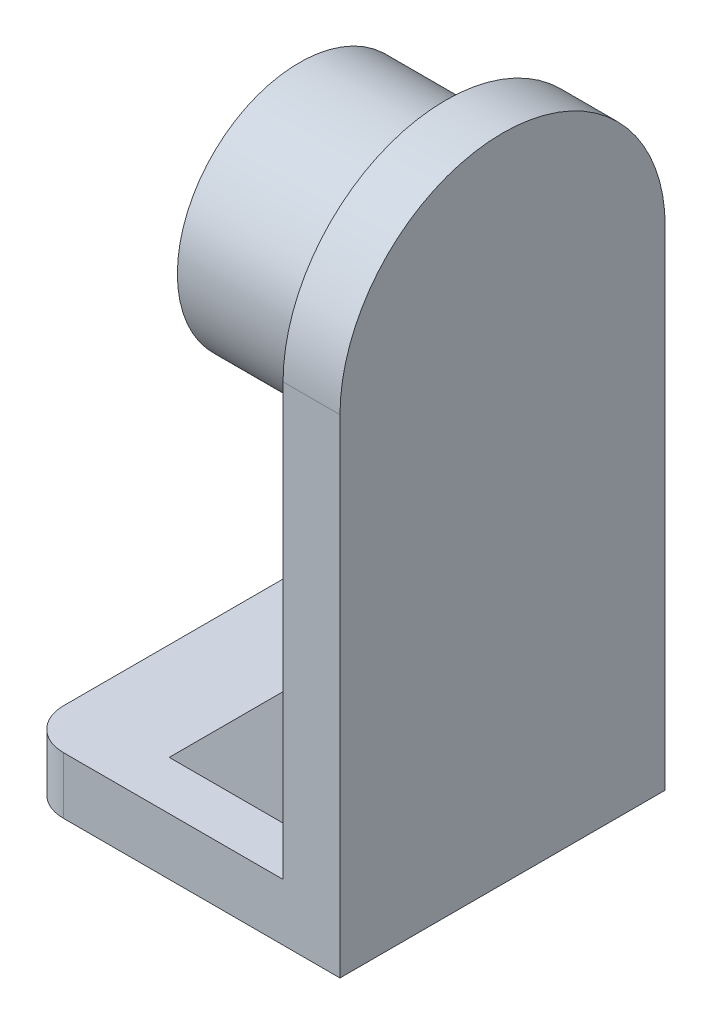
ISO-10303-21;
HEADER;
FILE_DESCRIPTION(('STEP AP214'),'2;1');
FILE_NAME('part.step','',(''),(''),'','','');
FILE_SCHEMA(('AUTOMOTIVE_DESIGN { 1 0 10303 214 1 1 1 1 }'));
ENDSEC;
DATA;
#1=APPLICATION_CONTEXT('core data for automotive mechanical design processes');
#2=APPLICATION_PROTOCOL_DEFINITION('international standard','automotive_design',2000,#1);
#3=PRODUCT_CONTEXT('',#1,'mechanical');
#4=PRODUCT('Part','Part','',(#3));
#5=PRODUCT_RELATED_PRODUCT_CATEGORY('part','',(#4));
#6=PRODUCT_DEFINITION_FORMATION('','',#4);
#7=PRODUCT_DEFINITION_CONTEXT('part definition',#1,'design');
#8=PRODUCT_DEFINITION('design','',#6,#7);
#9=PRODUCT_DEFINITION_SHAPE('','',#8);
#10=(LENGTH_UNIT() NAMED_UNIT(*) SI_UNIT(.MILLI.,.METRE.));
#11=(NAMED_UNIT(*) PLANE_ANGLE_UNIT() SI_UNIT($,.RADIAN.));
#12=(NAMED_UNIT(*) SI_UNIT($,.STERADIAN.) SOLID_ANGLE_UNIT());
#13=UNCERTAINTY_MEASURE_WITH_UNIT(LENGTH_MEASURE(1.E-05),#10,'distance_accuracy_value','');
#14=(GEOMETRIC_REPRESENTATION_CONTEXT(3) GLOBAL_UNCERTAINTY_ASSIGNED_CONTEXT((#13)) GLOBAL_UNIT_ASSIGNED_CONTEXT((#10,
#11,#12)) REPRESENTATION_CONTEXT('',''));
#15=CARTESIAN_POINT('',(0.,0.,0.));
#16=DIRECTION('',(0.,0.,1.));
#17=DIRECTION('',(1.,0.,0.));
#18=AXIS2_PLACEMENT_3D('',#15,#16,#17);
#19=CARTESIAN_POINT('',(7.,7.,12.));
#20=DIRECTION('',(-0.707106781186547,0.707106781186548,0.));
#21=DIRECTION('',(-0.707106781186548,-0.707106781186547,0.));
#22=AXIS2_PLACEMENT_3D('',#19,#20,#21);
#23=PLANE('',#22);
#24=DIRECTION('',(0.,0.,-1.));
#25=VECTOR('',#24,1.);
#26=CARTESIAN_POINT('',(27.,27.,12.));
#27=LINE('',#26,#25);
#28=CARTESIAN_POINT('',(27.,27.,12.));
#29=VERTEX_POINT('',#28);
#30=CARTESIAN_POINT('',(27.,27.,6.));
#31=VERTEX_POINT('',#30);
#32=EDGE_CURVE('E276',#29,#31,#27,.T.);
#33=ORIENTED_EDGE('',*,*,#32,.T.);
#34=DIRECTION('',(0.707106781186548,0.707106781186548,0.));
#35=VECTOR('',#34,1.);
#36=CARTESIAN_POINT('',(27.,27.,6.));
#37=LINE('',#36,#35);
#38=CARTESIAN_POINT('',(7.,7.,6.));
#39=VERTEX_POINT('',#38);
#40=EDGE_CURVE('E267',#39,#31,#37,.T.);
#41=ORIENTED_EDGE('',*,*,#40,.F.);
#42=DIRECTION('',(0.,0.,-1.));
#43=VECTOR('',#42,1.);
#44=CARTESIAN_POINT('',(7.,7.,12.));
#45=LINE('',#44,#43);
#46=CARTESIAN_POINT('',(7.,7.,12.));
#47=VERTEX_POINT('',#46);
#48=EDGE_CURVE('E279',#47,#39,#45,.T.);
#49=ORIENTED_EDGE('',*,*,#48,.F.);
#50=DIRECTION('',(0.707106781186548,0.707106781186547,0.));
#51=VECTOR('',#50,1.);
#52=CARTESIAN_POINT('',(7.,7.,12.));
#53=LINE('',#52,#51);
#54=EDGE_CURVE('E273',#47,#29,#53,.T.);
#55=ORIENTED_EDGE('',*,*,#54,.T.);
#56=EDGE_LOOP('',(#33,#41,#49,#55));
#57=FACE_BOUND('',#56,.T.);
#58=ADVANCED_FACE('F44',(#57),#23,.T.);
#59=CARTESIAN_POINT('',(0.,0.,40.));
#60=DIRECTION('',(0.,1.,0.));
#61=DIRECTION('',(0.,0.,1.));
#62=AXIS2_PLACEMENT_3D('',#59,#60,#61);
#63=PLANE('',#62);
#64=DIRECTION('',(1.,0.,0.));
#65=VECTOR('',#64,1.);
#66=CARTESIAN_POINT('',(0.,0.,0.));
#67=LINE('',#66,#65);
#68=CARTESIAN_POINT('',(0.,0.,0.));
#69=VERTEX_POINT('',#68);
#70=CARTESIAN_POINT('',(34.,0.,0.));
#71=VERTEX_POINT('',#70);
#72=EDGE_CURVE('E226',#69,#71,#67,.T.);
#73=ORIENTED_EDGE('',*,*,#72,.T.);
#74=DIRECTION('',(0.,0.,-1.));
#75=VECTOR('',#74,1.);
#76=CARTESIAN_POINT('',(34.,0.,40.));
#77=LINE('',#76,#75);
#78=CARTESIAN_POINT('',(34.,0.,40.));
#79=VERTEX_POINT('',#78);
#80=EDGE_CURVE('E52',#79,#71,#77,.T.);
#81=ORIENTED_EDGE('',*,*,#80,.F.);
#82=DIRECTION('',(1.,0.,0.));
#83=VECTOR('',#82,1.);
#84=CARTESIAN_POINT('',(0.,0.,40.));
#85=LINE('',#84,#83);
#86=CARTESIAN_POINT('',(0.,0.,40.));
#87=VERTEX_POINT('',#86);
#88=EDGE_CURVE('E211',#87,#79,#85,.T.);
#89=ORIENTED_EDGE('',*,*,#88,.F.);
#90=CARTESIAN_POINT('',(0.,0.,35.));
#91=DIRECTION('',(0.,1.,0.));
#92=DIRECTION('',(0.,0.,1.));
#93=AXIS2_PLACEMENT_3D('',#90,#91,#92);
#94=CIRCLE('',#93,5.);
#95=CARTESIAN_POINT('',(-5.,0.,35.));
#96=VERTEX_POINT('',#95);
#97=EDGE_CURVE('E196',#96,#87,#94,.T.);
#98=ORIENTED_EDGE('',*,*,#97,.F.);
#99=DIRECTION('',(0.,0.,1.));
#100=VECTOR('',#99,1.);
#101=CARTESIAN_POINT('',(-5.,0.,5.));
#102=LINE('',#101,#100);
#103=CARTESIAN_POINT('',(-5.,0.,5.));
#104=VERTEX_POINT('',#103);
#105=EDGE_CURVE('E195',#104,#96,#102,.T.);
#106=ORIENTED_EDGE('',*,*,#105,.F.);
#107=CARTESIAN_POINT('',(0.,0.,5.));
#108=DIRECTION('',(0.,1.,0.));
#109=DIRECTION('',(0.,0.,1.));
#110=AXIS2_PLACEMENT_3D('',#107,#108,#109);
#111=CIRCLE('',#110,5.);
#112=EDGE_CURVE('E186',#69,#104,#111,.T.);
#113=ORIENTED_EDGE('',*,*,#112,.F.);
#114=EDGE_LOOP('',(#73,#81,#89,#98,#106,#113));
#115=FACE_BOUND('',#114,.T.);
#116=ADVANCED_FACE('F50',(#115),#63,.F.);
#117=CARTESIAN_POINT('',(34.,0.,40.));
#118=DIRECTION('',(-1.,0.,0.));
#119=DIRECTION('',(0.,0.,1.));
#120=AXIS2_PLACEMENT_3D('',#117,#118,#119);
#121=PLANE('',#120);
#122=DIRECTION('',(0.,1.,0.));
#123=VECTOR('',#122,1.);
#124=CARTESIAN_POINT('',(34.,0.,0.));
#125=LINE('',#124,#123);
#126=CARTESIAN_POINT('',(34.,60.,0.));
#127=VERTEX_POINT('',#126);
#128=EDGE_CURVE('E229',#71,#127,#125,.T.);
#129=ORIENTED_EDGE('',*,*,#128,.T.);
#130=CARTESIAN_POINT('',(34.,60.,20.));
#131=DIRECTION('',(-1.,0.,0.));
#132=DIRECTION('',(0.,0.,1.));
#133=AXIS2_PLACEMENT_3D('',#130,#131,#132);
#134=CIRCLE('',#133,20.);
#135=CARTESIAN_POINT('',(34.,60.,40.));
#136=VERTEX_POINT('',#135);
#137=EDGE_CURVE('E182',#136,#127,#134,.T.);
#138=ORIENTED_EDGE('',*,*,#137,.F.);
#139=DIRECTION('',(0.,1.,0.));
#140=VECTOR('',#139,1.);
#141=CARTESIAN_POINT('',(34.,0.,40.));
#142=LINE('',#141,#140);
#143=EDGE_CURVE('E217',#79,#136,#142,.T.);
#144=ORIENTED_EDGE('',*,*,#143,.F.);
#145=ORIENTED_EDGE('',*,*,#80,.T.);
#146=EDGE_LOOP('',(#129,#138,#144,#145));
#147=FACE_BOUND('',#146,.T.);
#148=ADVANCED_FACE('F242',(#147),#121,.F.);
#149=CARTESIAN_POINT('',(27.,7.,40.));
#150=DIRECTION('',(1.,0.,0.));
#151=DIRECTION('',(0.,0.,-1.));
#152=AXIS2_PLACEMENT_3D('',#149,#150,#151);
#153=PLANE('',#152);
#154=CARTESIAN_POINT('',(27.,60.,20.));
#155=DIRECTION('',(1.,0.,0.));
#156=DIRECTION('',(0.,0.,-1.));
#157=AXIS2_PLACEMENT_3D('',#154,#155,#156);
#158=CIRCLE('',#157,15.);
#159=CARTESIAN_POINT('',(27.,60.,5.));
#160=VERTEX_POINT('',#159);
#161=EDGE_CURVE('E11',#160,#160,#158,.F.);
#162=ORIENTED_EDGE('',*,*,#161,.F.);
#163=EDGE_LOOP('',(#162));
#164=FACE_BOUND('',#163,.T.);
#165=DIRECTION('',(0.,-1.,0.));
#166=VECTOR('',#165,1.);
#167=CARTESIAN_POINT('',(27.,7.,0.));
#168=LINE('',#167,#166);
#169=CARTESIAN_POINT('',(27.,60.,0.));
#170=VERTEX_POINT('',#169);
#171=CARTESIAN_POINT('',(27.,7.,0.));
#172=VERTEX_POINT('',#171);
#173=EDGE_CURVE('E232',#170,#172,#168,.T.);
#174=ORIENTED_EDGE('',*,*,#173,.T.);
#175=DIRECTION('',(0.,0.,-1.));
#176=VECTOR('',#175,1.);
#177=CARTESIAN_POINT('',(27.,7.,6.));
#178=LINE('',#177,#176);
#179=CARTESIAN_POINT('',(27.,7.,6.));
#180=VERTEX_POINT('',#179);
#181=EDGE_CURVE('E269',#180,#172,#178,.T.);
#182=ORIENTED_EDGE('',*,*,#181,.F.);
#183=DIRECTION('',(0.,-1.,0.));
#184=VECTOR('',#183,1.);
#185=CARTESIAN_POINT('',(27.,7.,6.));
#186=LINE('',#185,#184);
#187=EDGE_CURVE('E261',#31,#180,#186,.T.);
#188=ORIENTED_EDGE('',*,*,#187,.F.);
#189=ORIENTED_EDGE('',*,*,#32,.F.);
#190=DIRECTION('',(0.,-1.,0.));
#191=VECTOR('',#190,1.);
#192=CARTESIAN_POINT('',(27.,27.,12.));
#193=LINE('',#192,#191);
#194=CARTESIAN_POINT('',(27.,7.,12.));
#195=VERTEX_POINT('',#194);
#196=EDGE_CURVE('E272',#29,#195,#193,.T.);
#197=ORIENTED_EDGE('',*,*,#196,.T.);
#198=DIRECTION('',(0.,0.,-1.));
#199=VECTOR('',#198,1.);
#200=CARTESIAN_POINT('',(27.,7.,40.));
#201=LINE('',#200,#199);
#202=CARTESIAN_POINT('',(27.,7.,28.));
#203=VERTEX_POINT('',#202);
#204=EDGE_CURVE('E223',#203,#195,#201,.T.);
#205=ORIENTED_EDGE('',*,*,#204,.F.);
#206=DIRECTION('',(0.,1.,0.));
#207=VECTOR('',#206,1.);
#208=CARTESIAN_POINT('',(27.,7.,28.));
#209=LINE('',#208,#207);
#210=CARTESIAN_POINT('',(27.,27.,28.));
#211=VERTEX_POINT('',#210);
#212=EDGE_CURVE('E285',#203,#211,#209,.T.);
#213=ORIENTED_EDGE('',*,*,#212,.T.);
#214=DIRECTION('',(0.,0.,1.));
#215=VECTOR('',#214,1.);
#216=CARTESIAN_POINT('',(27.,27.,28.));
#217=LINE('',#216,#215);
#218=CARTESIAN_POINT('',(27.,27.,34.));
#219=VERTEX_POINT('',#218);
#220=EDGE_CURVE('E166',#211,#219,#217,.T.);
#221=ORIENTED_EDGE('',*,*,#220,.T.);
#222=DIRECTION('',(0.,1.,0.));
#223=VECTOR('',#222,1.);
#224=CARTESIAN_POINT('',(27.,7.,34.));
#225=LINE('',#224,#223);
#226=CARTESIAN_POINT('',(27.,7.,34.));
#227=VERTEX_POINT('',#226);
#228=EDGE_CURVE('E58',#227,#219,#225,.T.);
#229=ORIENTED_EDGE('',*,*,#228,.F.);
#230=DIRECTION('',(0.,0.,1.));
#231=VECTOR('',#230,1.);
#232=CARTESIAN_POINT('',(27.,7.,34.));
#233=LINE('',#232,#231);
#234=CARTESIAN_POINT('',(27.,7.,40.));
#235=VERTEX_POINT('',#234);
#236=EDGE_CURVE('E163',#227,#235,#233,.T.);
#237=ORIENTED_EDGE('',*,*,#236,.T.);
#238=DIRECTION('',(0.,-1.,0.));
#239=VECTOR('',#238,1.);
#240=CARTESIAN_POINT('',(27.,7.,40.));
#241=LINE('',#240,#239);
#242=CARTESIAN_POINT('',(27.,60.,40.));
#243=VERTEX_POINT('',#242);
#244=EDGE_CURVE('E222',#243,#235,#241,.T.);
#245=ORIENTED_EDGE('',*,*,#244,.F.);
#246=CARTESIAN_POINT('',(27.,60.,20.));
#247=DIRECTION('',(-1.,0.,0.));
#248=DIRECTION('',(0.,0.,1.));
#249=AXIS2_PLACEMENT_3D('',#246,#247,#248);
#250=CIRCLE('',#249,20.);
#251=EDGE_CURVE('E185',#243,#170,#250,.T.);
#252=ORIENTED_EDGE('',*,*,#251,.T.);
#253=EDGE_LOOP('',(#174,#182,#188,#189,#197,#205,#213,#221,#229,#237,#245,#252));
#254=FACE_BOUND('',#253,.T.);
#255=ADVANCED_FACE('F258',(#164,#254),#153,.F.);
#256=CARTESIAN_POINT('',(0.,7.,40.));
#257=DIRECTION('',(0.,-1.,0.));
#258=DIRECTION('',(0.,0.,-1.));
#259=AXIS2_PLACEMENT_3D('',#256,#257,#258);
#260=PLANE('',#259);
#261=DIRECTION('',(-1.,0.,0.));
#262=VECTOR('',#261,1.);
#263=CARTESIAN_POINT('',(27.,7.,12.));
#264=LINE('',#263,#262);
#265=EDGE_CURVE('E271',#195,#47,#264,.T.);
#266=ORIENTED_EDGE('',*,*,#265,.T.);
#267=ORIENTED_EDGE('',*,*,#48,.T.);
#268=DIRECTION('',(-1.,0.,0.));
#269=VECTOR('',#268,1.);
#270=CARTESIAN_POINT('',(7.,7.,6.));
#271=LINE('',#270,#269);
#272=EDGE_CURVE('E69',#180,#39,#271,.T.);
#273=ORIENTED_EDGE('',*,*,#272,.F.);
#274=ORIENTED_EDGE('',*,*,#181,.T.);
#275=DIRECTION('',(-1.,0.,0.));
#276=VECTOR('',#275,1.);
#277=CARTESIAN_POINT('',(0.,7.,0.));
#278=LINE('',#277,#276);
#279=CARTESIAN_POINT('',(0.,7.,0.));
#280=VERTEX_POINT('',#279);
#281=EDGE_CURVE('E213',#172,#280,#278,.T.);
#282=ORIENTED_EDGE('',*,*,#281,.T.);
#283=CARTESIAN_POINT('',(0.,7.,5.));
#284=DIRECTION('',(0.,1.,0.));
#285=DIRECTION('',(0.,0.,1.));
#286=AXIS2_PLACEMENT_3D('',#283,#284,#285);
#287=CIRCLE('',#286,5.);
#288=CARTESIAN_POINT('',(-5.,7.,5.));
#289=VERTEX_POINT('',#288);
#290=EDGE_CURVE('E187',#280,#289,#287,.T.);
#291=ORIENTED_EDGE('',*,*,#290,.T.);
#292=DIRECTION('',(0.,0.,1.));
#293=VECTOR('',#292,1.);
#294=CARTESIAN_POINT('',(-5.,7.,5.));
#295=LINE('',#294,#293);
#296=CARTESIAN_POINT('',(-5.,7.,35.));
#297=VERTEX_POINT('',#296);
#298=EDGE_CURVE('E205',#289,#297,#295,.T.);
#299=ORIENTED_EDGE('',*,*,#298,.T.);
#300=CARTESIAN_POINT('',(0.,7.,35.));
#301=DIRECTION('',(0.,1.,0.));
#302=DIRECTION('',(0.,0.,1.));
#303=AXIS2_PLACEMENT_3D('',#300,#301,#302);
#304=CIRCLE('',#303,5.);
#305=CARTESIAN_POINT('',(0.,7.,40.));
#306=VERTEX_POINT('',#305);
#307=EDGE_CURVE('E194',#297,#306,#304,.T.);
#308=ORIENTED_EDGE('',*,*,#307,.T.);
#309=DIRECTION('',(-1.,0.,0.));
#310=VECTOR('',#309,1.);
#311=CARTESIAN_POINT('',(0.,7.,40.));
#312=LINE('',#311,#310);
#313=EDGE_CURVE('E224',#235,#306,#312,.T.);
#314=ORIENTED_EDGE('',*,*,#313,.F.);
#315=ORIENTED_EDGE('',*,*,#236,.F.);
#316=DIRECTION('',(1.,0.,0.));
#317=VECTOR('',#316,1.);
#318=CARTESIAN_POINT('',(7.,7.,34.));
#319=LINE('',#318,#317);
#320=CARTESIAN_POINT('',(7.,7.,34.));
#321=VERTEX_POINT('',#320);
#322=EDGE_CURVE('E146',#321,#227,#319,.T.);
#323=ORIENTED_EDGE('',*,*,#322,.F.);
#324=DIRECTION('',(0.,0.,1.));
#325=VECTOR('',#324,1.);
#326=CARTESIAN_POINT('',(7.,7.,28.));
#327=LINE('',#326,#325);
#328=CARTESIAN_POINT('',(7.,7.,28.));
#329=VERTEX_POINT('',#328);
#330=EDGE_CURVE('E159',#329,#321,#327,.T.);
#331=ORIENTED_EDGE('',*,*,#330,.F.);
#332=DIRECTION('',(1.,0.,0.));
#333=VECTOR('',#332,1.);
#334=CARTESIAN_POINT('',(27.,7.,28.));
#335=LINE('',#334,#333);
#336=EDGE_CURVE('E282',#329,#203,#335,.T.);
#337=ORIENTED_EDGE('',*,*,#336,.T.);
#338=ORIENTED_EDGE('',*,*,#204,.T.);
#339=EDGE_LOOP('',(#266,#267,#273,#274,#282,#291,#299,#308,#314,#315,#323,#331,#337,#338));
#340=FACE_BOUND('',#339,.T.);
#341=ADVANCED_FACE('F157',(#340),#260,.F.);
#342=CARTESIAN_POINT('',(0.,0.,40.));
#343=DIRECTION('',(0.,0.,-1.));
#344=DIRECTION('',(-1.,0.,0.));
#345=AXIS2_PLACEMENT_3D('',#342,#343,#344);
#346=PLANE('',#345);
#347=ORIENTED_EDGE('',*,*,#244,.T.);
#348=ORIENTED_EDGE('',*,*,#313,.T.);
#349=DIRECTION('',(0.,-1.,0.));
#350=VECTOR('',#349,1.);
#351=CARTESIAN_POINT('',(0.,0.,40.));
#352=LINE('',#351,#350);
#353=EDGE_CURVE('E212',#306,#87,#352,.T.);
#354=ORIENTED_EDGE('',*,*,#353,.T.);
#355=ORIENTED_EDGE('',*,*,#88,.T.);
#356=ORIENTED_EDGE('',*,*,#143,.T.);
#357=DIRECTION('',(-1.,0.,0.));
#358=VECTOR('',#357,1.);
#359=CARTESIAN_POINT('',(34.,60.,40.));
#360=LINE('',#359,#358);
#361=EDGE_CURVE('E218',#136,#243,#360,.T.);
#362=ORIENTED_EDGE('',*,*,#361,.T.);
#363=EDGE_LOOP('',(#347,#348,#354,#355,#356,#362));
#364=FACE_BOUND('',#363,.T.);
#365=ADVANCED_FACE('F259',(#364),#346,.F.);
#366=CARTESIAN_POINT('',(0.,0.,0.));
#367=DIRECTION('',(0.,0.,-1.));
#368=DIRECTION('',(-1.,0.,0.));
#369=AXIS2_PLACEMENT_3D('',#366,#367,#368);
#370=PLANE('',#369);
#371=ORIENTED_EDGE('',*,*,#281,.F.);
#372=ORIENTED_EDGE('',*,*,#173,.F.);
#373=DIRECTION('',(-1.,0.,0.));
#374=VECTOR('',#373,1.);
#375=CARTESIAN_POINT('',(34.,60.,0.));
#376=LINE('',#375,#374);
#377=EDGE_CURVE('E235',#127,#170,#376,.T.);
#378=ORIENTED_EDGE('',*,*,#377,.F.);
#379=ORIENTED_EDGE('',*,*,#128,.F.);
#380=ORIENTED_EDGE('',*,*,#72,.F.);
#381=DIRECTION('',(0.,-1.,0.));
#382=VECTOR('',#381,1.);
#383=CARTESIAN_POINT('',(0.,0.,0.));
#384=LINE('',#383,#382);
#385=EDGE_CURVE('E209',#280,#69,#384,.T.);
#386=ORIENTED_EDGE('',*,*,#385,.F.);
#387=EDGE_LOOP('',(#371,#372,#378,#379,#380,#386));
#388=FACE_BOUND('',#387,.T.);
#389=ADVANCED_FACE('F249',(#388),#370,.T.);
#390=CARTESIAN_POINT('',(0.,0.,5.));
#391=DIRECTION('',(0.,1.,0.));
#392=DIRECTION('',(0.,0.,1.));
#393=AXIS2_PLACEMENT_3D('',#390,#391,#392);
#394=CYLINDRICAL_SURFACE('',#393,5.);
#395=ORIENTED_EDGE('',*,*,#290,.F.);
#396=ORIENTED_EDGE('',*,*,#385,.T.);
#397=ORIENTED_EDGE('',*,*,#112,.T.);
#398=DIRECTION('',(0.,1.,0.));
#399=VECTOR('',#398,1.);
#400=CARTESIAN_POINT('',(-5.,0.,5.));
#401=LINE('',#400,#399);
#402=EDGE_CURVE('E198',#104,#289,#401,.T.);
#403=ORIENTED_EDGE('',*,*,#402,.T.);
#404=EDGE_LOOP('',(#395,#396,#397,#403));
#405=FACE_BOUND('',#404,.T.);
#406=ADVANCED_FACE('F301',(#405),#394,.T.);
#407=CARTESIAN_POINT('',(0.,0.,35.));
#408=DIRECTION('',(0.,1.,0.));
#409=DIRECTION('',(0.,0.,1.));
#410=AXIS2_PLACEMENT_3D('',#407,#408,#409);
#411=CYLINDRICAL_SURFACE('',#410,5.);
#412=ORIENTED_EDGE('',*,*,#307,.F.);
#413=DIRECTION('',(0.,1.,0.));
#414=VECTOR('',#413,1.);
#415=CARTESIAN_POINT('',(-5.,0.,35.));
#416=LINE('',#415,#414);
#417=EDGE_CURVE('E210',#96,#297,#416,.T.);
#418=ORIENTED_EDGE('',*,*,#417,.F.);
#419=ORIENTED_EDGE('',*,*,#97,.T.);
#420=ORIENTED_EDGE('',*,*,#353,.F.);
#421=EDGE_LOOP('',(#412,#418,#419,#420));
#422=FACE_BOUND('',#421,.T.);
#423=ADVANCED_FACE('F309',(#422),#411,.T.);
#424=CARTESIAN_POINT('',(-5.,0.,5.));
#425=DIRECTION('',(-1.,0.,0.));
#426=DIRECTION('',(0.,0.,1.));
#427=AXIS2_PLACEMENT_3D('',#424,#425,#426);
#428=PLANE('',#427);
#429=ORIENTED_EDGE('',*,*,#298,.F.);
#430=ORIENTED_EDGE('',*,*,#402,.F.);
#431=ORIENTED_EDGE('',*,*,#105,.T.);
#432=ORIENTED_EDGE('',*,*,#417,.T.);
#433=EDGE_LOOP('',(#429,#430,#431,#432));
#434=FACE_BOUND('',#433,.T.);
#435=ADVANCED_FACE('F304',(#434),#428,.T.);
#436=CARTESIAN_POINT('',(34.,60.,20.));
#437=DIRECTION('',(-1.,0.,0.));
#438=DIRECTION('',(0.,0.,1.));
#439=AXIS2_PLACEMENT_3D('',#436,#437,#438);
#440=CYLINDRICAL_SURFACE('',#439,20.);
#441=ORIENTED_EDGE('',*,*,#251,.F.);
#442=ORIENTED_EDGE('',*,*,#361,.F.);
#443=ORIENTED_EDGE('',*,*,#137,.T.);
#444=ORIENTED_EDGE('',*,*,#377,.T.);
#445=EDGE_LOOP('',(#441,#442,#443,#444));
#446=FACE_BOUND('',#445,.T.);
#447=ADVANCED_FACE('F253',(#446),#440,.T.);
#448=CARTESIAN_POINT('',(9.00000000000001,60.,20.));
#449=DIRECTION('',(1.,0.,0.));
#450=DIRECTION('',(0.,0.,-1.));
#451=AXIS2_PLACEMENT_3D('',#448,#449,#450);
#452=CYLINDRICAL_SURFACE('',#451,15.);
#453=CARTESIAN_POINT('',(9.00000000000001,60.,20.));
#454=DIRECTION('',(-1.,0.,0.));
#455=DIRECTION('',(0.,0.,1.));
#456=AXIS2_PLACEMENT_3D('',#453,#454,#455);
#457=CIRCLE('',#456,15.);
#458=CARTESIAN_POINT('',(9.00000000000001,60.,35.));
#459=VERTEX_POINT('',#458);
#460=EDGE_CURVE('E178',#459,#459,#457,.T.);
#461=ORIENTED_EDGE('',*,*,#460,.F.);
#462=EDGE_LOOP('',(#461));
#463=FACE_BOUND('',#462,.T.);
#464=ORIENTED_EDGE('',*,*,#161,.T.);
#465=EDGE_LOOP('',(#464));
#466=FACE_BOUND('',#465,.T.);
#467=ADVANCED_FACE('F339',(#463,#466),#452,.T.);
#468=CARTESIAN_POINT('',(9.00000000000001,60.,20.));
#469=DIRECTION('',(-1.,0.,0.));
#470=DIRECTION('',(0.,0.,1.));
#471=AXIS2_PLACEMENT_3D('',#468,#469,#470);
#472=PLANE('',#471);
#473=CARTESIAN_POINT('',(9.00000000000001,60.,20.));
#474=DIRECTION('',(-1.,0.,0.));
#475=DIRECTION('',(0.,0.,1.));
#476=AXIS2_PLACEMENT_3D('',#473,#474,#475);
#477=CIRCLE('',#476,11.);
#478=CARTESIAN_POINT('',(9.00000000000001,60.,31.));
#479=VERTEX_POINT('',#478);
#480=EDGE_CURVE('E170',#479,#479,#477,.T.);
#481=ORIENTED_EDGE('',*,*,#480,.F.);
#482=EDGE_LOOP('',(#481));
#483=FACE_BOUND('',#482,.T.);
#484=ORIENTED_EDGE('',*,*,#460,.T.);
#485=EDGE_LOOP('',(#484));
#486=FACE_BOUND('',#485,.T.);
#487=ADVANCED_FACE('F333',(#483,#486),#472,.T.);
#488=CARTESIAN_POINT('',(27.,60.,20.));
#489=DIRECTION('',(-1.,0.,0.));
#490=DIRECTION('',(0.,0.,1.));
#491=AXIS2_PLACEMENT_3D('',#488,#489,#490);
#492=CYLINDRICAL_SURFACE('',#491,11.);
#493=CARTESIAN_POINT('',(27.,60.,20.));
#494=DIRECTION('',(-1.,0.,0.));
#495=DIRECTION('',(0.,0.,1.));
#496=AXIS2_PLACEMENT_3D('',#493,#494,#495);
#497=CIRCLE('',#496,11.);
#498=CARTESIAN_POINT('',(27.,60.,31.));
#499=VERTEX_POINT('',#498);
#500=EDGE_CURVE('E171',#499,#499,#497,.T.);
#501=ORIENTED_EDGE('',*,*,#500,.F.);
#502=EDGE_LOOP('',(#501));
#503=FACE_BOUND('',#502,.T.);
#504=ORIENTED_EDGE('',*,*,#480,.T.);
#505=EDGE_LOOP('',(#504));
#506=FACE_BOUND('',#505,.T.);
#507=ADVANCED_FACE('F332',(#503,#506),#492,.F.);
#508=CARTESIAN_POINT('',(27.,60.,20.));
#509=DIRECTION('',(-1.,0.,0.));
#510=DIRECTION('',(0.,0.,1.));
#511=AXIS2_PLACEMENT_3D('',#508,#509,#510);
#512=PLANE('',#511);
#513=ORIENTED_EDGE('',*,*,#500,.T.);
#514=EDGE_LOOP('',(#513));
#515=FACE_BOUND('',#514,.T.);
#516=ADVANCED_FACE('F329',(#515),#512,.T.);
#517=CARTESIAN_POINT('',(7.,7.,28.));
#518=DIRECTION('',(-0.707106781186547,0.707106781186548,0.));
#519=DIRECTION('',(-0.707106781186548,-0.707106781186547,0.));
#520=AXIS2_PLACEMENT_3D('',#517,#518,#519);
#521=PLANE('',#520);
#522=DIRECTION('',(-0.707106781186548,-0.707106781186547,0.));
#523=VECTOR('',#522,1.);
#524=CARTESIAN_POINT('',(27.,27.,34.));
#525=LINE('',#524,#523);
#526=EDGE_CURVE('E147',#219,#321,#525,.T.);
#527=ORIENTED_EDGE('',*,*,#526,.F.);
#528=ORIENTED_EDGE('',*,*,#220,.F.);
#529=DIRECTION('',(-0.707106781186548,-0.707106781186547,0.));
#530=VECTOR('',#529,1.);
#531=CARTESIAN_POINT('',(7.,7.,28.));
#532=LINE('',#531,#530);
#533=EDGE_CURVE('E168',#211,#329,#532,.T.);
#534=ORIENTED_EDGE('',*,*,#533,.T.);
#535=ORIENTED_EDGE('',*,*,#330,.T.);
#536=EDGE_LOOP('',(#527,#528,#534,#535));
#537=FACE_BOUND('',#536,.T.);
#538=ADVANCED_FACE('F165',(#537),#521,.T.);
#539=CARTESIAN_POINT('',(0.,0.,28.));
#540=DIRECTION('',(0.,0.,-1.));
#541=DIRECTION('',(-1.,0.,0.));
#542=AXIS2_PLACEMENT_3D('',#539,#540,#541);
#543=PLANE('',#542);
#544=ORIENTED_EDGE('',*,*,#336,.F.);
#545=ORIENTED_EDGE('',*,*,#533,.F.);
#546=ORIENTED_EDGE('',*,*,#212,.F.);
#547=EDGE_LOOP('',(#544,#545,#546));
#548=FACE_BOUND('',#547,.T.);
#549=ADVANCED_FACE('F286',(#548),#543,.T.);
#550=CARTESIAN_POINT('',(0.,0.,12.));
#551=DIRECTION('',(0.,0.,-1.));
#552=DIRECTION('',(-1.,0.,0.));
#553=AXIS2_PLACEMENT_3D('',#550,#551,#552);
#554=PLANE('',#553);
#555=ORIENTED_EDGE('',*,*,#196,.F.);
#556=ORIENTED_EDGE('',*,*,#54,.F.);
#557=ORIENTED_EDGE('',*,*,#265,.F.);
#558=EDGE_LOOP('',(#555,#556,#557));
#559=FACE_BOUND('',#558,.T.);
#560=ADVANCED_FACE('F294',(#559),#554,.F.);
#561=CARTESIAN_POINT('',(0.,0.,6.));
#562=DIRECTION('',(0.,0.,-1.));
#563=DIRECTION('',(-1.,0.,0.));
#564=AXIS2_PLACEMENT_3D('',#561,#562,#563);
#565=PLANE('',#564);
#566=ORIENTED_EDGE('',*,*,#187,.T.);
#567=ORIENTED_EDGE('',*,*,#272,.T.);
#568=ORIENTED_EDGE('',*,*,#40,.T.);
#569=EDGE_LOOP('',(#566,#567,#568));
#570=FACE_BOUND('',#569,.T.);
#571=ADVANCED_FACE('F300',(#570),#565,.T.);
#572=CARTESIAN_POINT('',(0.,0.,34.));
#573=DIRECTION('',(0.,0.,-1.));
#574=DIRECTION('',(-1.,0.,0.));
#575=AXIS2_PLACEMENT_3D('',#572,#573,#574);
#576=PLANE('',#575);
#577=ORIENTED_EDGE('',*,*,#228,.T.);
#578=ORIENTED_EDGE('',*,*,#526,.T.);
#579=ORIENTED_EDGE('',*,*,#322,.T.);
#580=EDGE_LOOP('',(#577,#578,#579));
#581=FACE_BOUND('',#580,.T.);
#582=ADVANCED_FACE('F149',(#581),#576,.F.);
#583=CLOSED_SHELL('',(#58,#116,#148,#255,#341,#365,#389,#406,#423,#435,#447,#467,#487,#507,#516,
#538,#549,#560,#571,#582));
#584=MANIFOLD_SOLID_BREP('B2',#583);
#585=ADVANCED_BREP_SHAPE_REPRESENTATION('',(#18,#584),#14);
#586=SHAPE_DEFINITION_REPRESENTATION(#9,#585);
ENDSEC;
END-ISO-10303-21;
